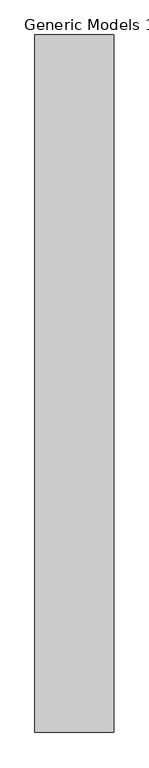
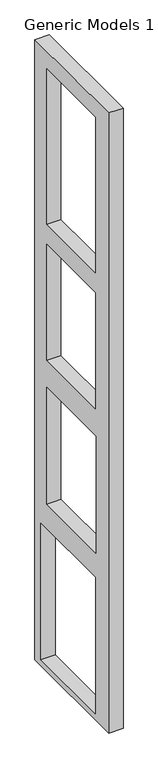
"""IFC4 building model written with IfcOpenShell, lengths in millimetres: proxy geometry, Generic Models 1 : Generic Models 1."""

from ifc_helpers import new_model, si_unit, frame, origin, place, context, project, spatial, polyline, outline, extrude, source, transform, mapped, element, save


def generic_models_1_generic_models_1_8cf75778(model_context):
    return source(origin(), model_context, "Body", "SweptSolid", [
        extrude(outline(polyline([(-1163.3455717, 13106.4), (1412.8547293, 13106.4), (1412.8547293, -120.3784961), (-1163.3455717, -120.3784961), (-1163.3455717, 13106.4)]), holes=[polyline([(1006.4547293, 9414.8838451), (1006.4547293, 12728.4662996), (-695.3452707, 12728.4662996), (-695.3452707, 9414.8838451), (1006.4547293, 9414.8838451)]), polyline([(1006.4547293, 6512.1761812), (1006.4547293, 8991.6), (-695.3452707, 8991.6), (-695.3452707, 6512.1761812), (1006.4547293, 6512.1761812)]), polyline([(1006.4547293, 3444.7360251), (1006.4547293, 5943.6), (-714.2964201, 5943.6), (-714.2964201, 3444.7360251), (1006.4547293, 3444.7360251)]), polyline([(1209.6547293, 5.5533975), (1209.6547293, 2920.053109), (-695.3452707, 2920.053109), (-695.3452707, 5.5533975), (1209.6547293, 5.5533975)])]), frame((5029.6941283, 0.0, 0.0), z_axis=(1.0, 0.0, 0.0), x_axis=(0.0, 1.0, 0.0)), (0.0, 0.0, 1.0), 291.235164),
    ])


if __name__ == "__main__":
    model = new_model("IFC4")
    model_context = context("Model", 3, world=origin())
    ifc_project = project(units=[si_unit("LENGTHUNIT", "METRE", prefix="MILLI")], contexts=[model_context])
    site = spatial("IfcSite", under=ifc_project)
    building = spatial("IfcBuilding", under=site)
    placement = place(None, origin())
    generic_models_1_generic_models_1_shape = generic_models_1_generic_models_1_8cf75778(model_context)
    element("IfcBuildingElementProxy", 1, Name="Generic Models 1 : Generic Models 1", ObjectType="Generic Models 1 : Generic Models 1", at=placement, inside=building, context=model_context, shape_type="MappedRepresentation", body=[
        mapped(generic_models_1_generic_models_1_shape, transform((0.0, 0.0, 0.0), x_axis=(1.0, 0.0, 0.0), y_axis=(0.0, 1.0, 0.0), z_axis=(0.0, 0.0, 1.0))),
    ])
    save(model, "model.ifc")

# Revit data of these elements
# Element 1 (IfcBuildingElementProxy, "Generic Models 1 : Generic Models 1")
#   Materials on its faces: "Acoustic Ceiling Tile 24 x 24", "Door - Frame"
# Materials
#   "Acoustic Ceiling Tile 24 x 24": class "Generic", colour RGB 232 232 232, transparency 0, Description = "Acoustic Ceiling Tile 24 x 24", Cost = 0
#   "Door - Frame": colour RGB 118 70 51, transparency 0, Cost = 0
